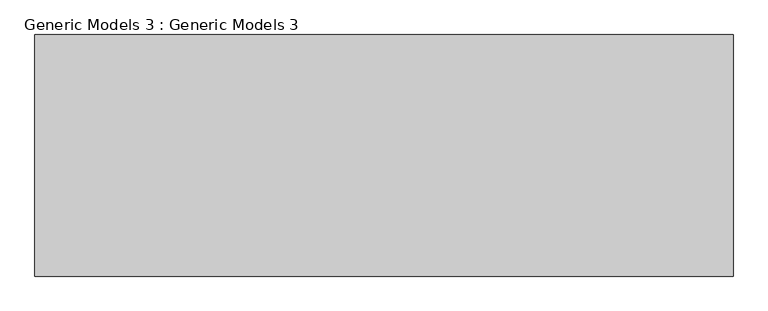
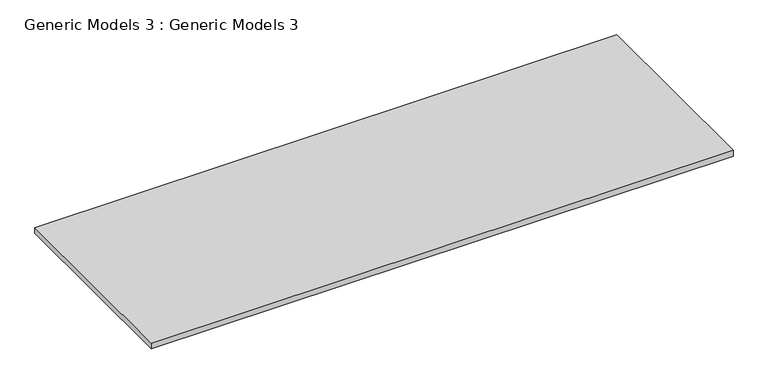
"""IFC4 building model written with IfcOpenShell, lengths in millimetres: proxy geometry, Generic Models 3 : Generic Models 3."""

from ifc_helpers import new_model, si_unit, frame, origin, place, context, project, spatial, polyline, outline, extrude, source, transform, mapped, element, save


def generic_models_3_generic_models_3_7537cf84(model_context):
    return source(origin(), model_context, "Body", "SweptSolid", [
        extrude(outline(polyline([(-8698.9796736, -8350.9396544), (5931.4203264, -8350.9396544), (5931.4203264, -13415.3421778), (-8698.9796736, -13415.3421778), (-8698.9796736, -8350.9396544)])), frame((0.0, 0.0, -152.4), z_axis=(0.0, 0.0, 1.0), x_axis=(1.0, 0.0, 0.0)), (0.0, 0.0, 1.0), 152.4),
    ])


if __name__ == "__main__":
    model = new_model("IFC4")
    model_context = context("Model", 3, world=origin())
    ifc_project = project(units=[si_unit("LENGTHUNIT", "METRE", prefix="MILLI")], contexts=[model_context])
    site = spatial("IfcSite", under=ifc_project)
    building = spatial("IfcBuilding", under=site)
    placement = place(None, origin())
    generic_models_3_generic_models_3_shape = generic_models_3_generic_models_3_7537cf84(model_context)
    element("IfcBuildingElementProxy", 1, Name="Generic Models 3 : Generic Models 3", ObjectType="Generic Models 3 : Generic Models 3", at=placement, inside=building, context=model_context, shape_type="MappedRepresentation", body=[
        mapped(generic_models_3_generic_models_3_shape, transform((0.0, 0.0, 0.0), x_axis=(1.0, 0.0, 0.0), y_axis=(0.0, 1.0, 0.0), z_axis=(0.0, 0.0, 1.0))),
    ])
    save(model, "model.ifc")
